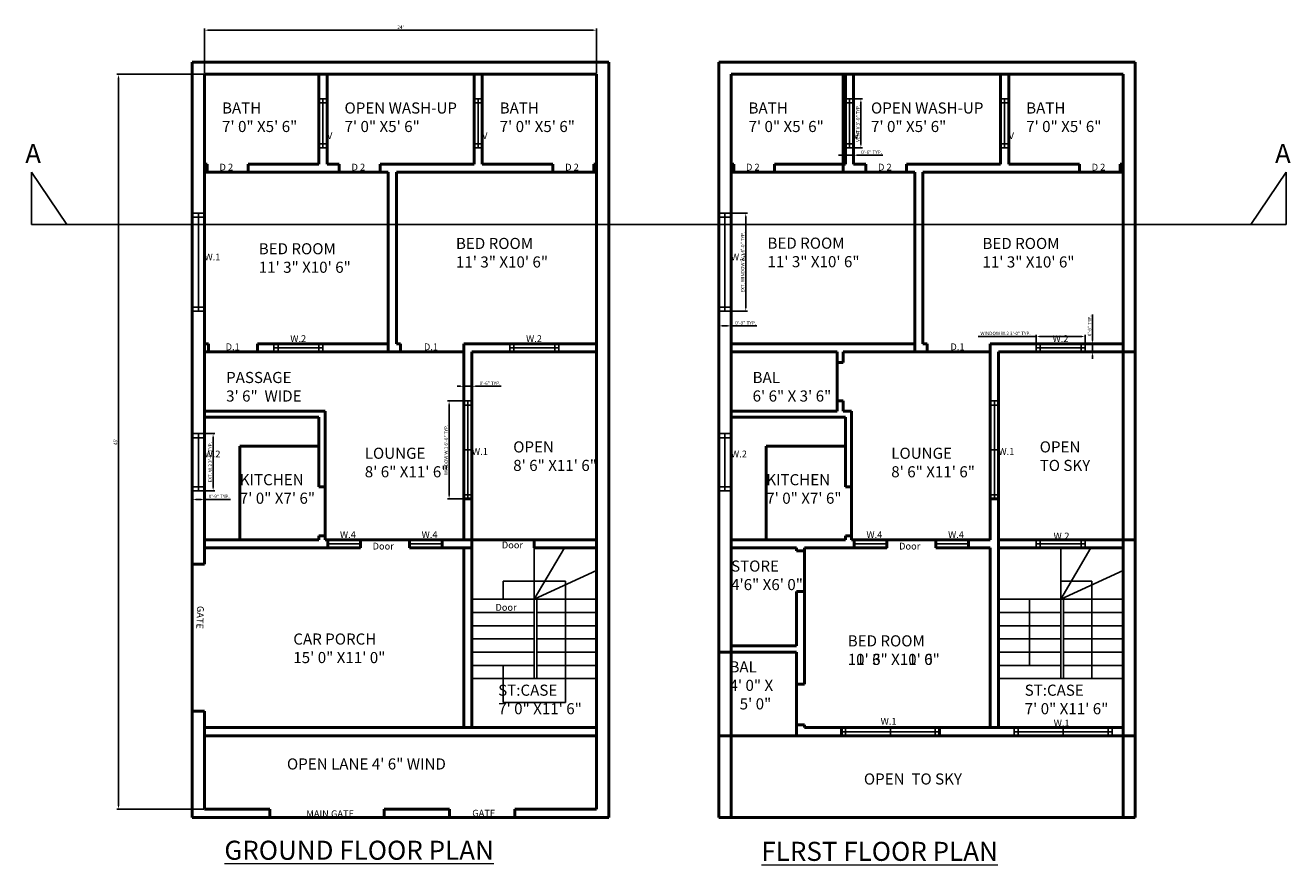
# Model space of a CAD drawing. Units: inches. Extents: x 2117 to 3047, y 1240 to 2266.
# Tile 1 of 4: x 2117 to 3047, y 1240 to 1856. Entities that reach past the tile are written whole.
import ezdxf

# ---------------------------------------------------------------- set-up
doc = ezdxf.new("R2010")
doc.units = ezdxf.units.IN
for name, color, linetype, lineweight in [('A-ANNO-DIMS', 2, 'Continuous', 18), ('A-ANNO-SYMB', 1, 'Continuous', 25), ('A-ANNO-TEXT', 7, 'Continuous', 18), ('A-AREA-IDEN', 3, 'Continuous', 18), ('A-FLOR-STRS', 51, 'Continuous', 25), ('A-GLAZ', 4, 'Continuous', 25), ('A-WALL', 7, 'Continuous', 50)]:
    doc.layers.add(name, color=color, linetype=linetype, lineweight=lineweight)
doc.styles.get("Standard").update_dxf_attribs({"font": 'arial.ttf'})
doc.dimstyles.new('ISO-25', dxfattribs={"dimtxt": 2.5, "dimasz": 2.5, "dimexe": 1.25, "dimexo": 0.625, "dimtad": 1, "dimdec": 1, "dimlunit": 3, "dimtxsty": 'Standard', "dimcen": 2.5, "dimadec": 0, "dimazin": 0, "dimtfac": 1, "dimtdec": 1, "dimtmove": 0, "dimatfit": 3, "dimfxl": 1, "dimarcsym": 0})

# ---------------------------------------------------------------- blocks, each defined once
blk = doc.blocks.new('*D1')
at = {"layer": 'A-ANNO-DIMS', "color": 0, "lineweight": -2, "transparency": 16777216}
for p, q in [((2249.01, 1820.83), (2249.01, 1853.88)), ((2534.51, 1852.63), (2251.51, 1852.63)), ((2537.01, 1820.83), (2537.01, 1853.88))]:
    blk.add_line(p, q, dxfattribs=at)
at = {"layer": 'A-ANNO-DIMS', "color": 0, "transparency": 16777216}
for points in [[(2251.51, 1853.05), (2251.51, 1852.21), (2249.01, 1852.63)], [(2534.51, 1853.05), (2534.51, 1852.21), (2537.01, 1852.63)]]:
    blk.add_solid(points, dxfattribs=at)
at = {"layer": 'Defpoints', "color": 0, "transparency": 16777216}
for p in [(2249.01, 1852.63), (2249.01, 1820.2), (2537.01, 1820.2)]:
    blk.add_point(p, dxfattribs=at)
at = {"layer": 'A-ANNO-DIMS', "color": 0, "transparency": 16777216, "insert": (2393.01, 1854.51), "char_height": 2.5, "attachment_point": 5}
blk.add_mtext("24'", dxfattribs=at)
blk = doc.blocks.new('*D2')
at = {"layer": 'A-ANNO-DIMS', "color": 0, "lineweight": -2, "transparency": 16777216}
for p, q in [((2248.39, 1820.2), (2184.53, 1820.2)), ((2185.78, 1817.7), (2185.78, 1282.7)), ((2248.39, 1280.2), (2184.53, 1280.2))]:
    blk.add_line(p, q, dxfattribs=at)
at = {"layer": 'A-ANNO-DIMS', "color": 0, "transparency": 16777216}
for points in [[(2185.36, 1817.7), (2186.19, 1817.7), (2185.78, 1820.2)], [(2185.36, 1282.7), (2186.19, 1282.7), (2185.78, 1280.2)]]:
    blk.add_solid(points, dxfattribs=at)
at = {"layer": 'Defpoints', "color": 0, "transparency": 16777216}
for p in [(2249.01, 1820.2), (2185.78, 1280.2), (2249.01, 1280.2)]:
    blk.add_point(p, dxfattribs=at)
at = {"layer": 'A-ANNO-DIMS', "color": 0, "transparency": 16777216, "insert": (2183.88, 1550.2), "char_height": 2.5, "attachment_point": 5, "rotation": 90}
blk.add_mtext("45'", dxfattribs=at)
blk = doc.blocks.new('WIN-36')
for p, q in [((0, 36), (6, 36)), ((6, 36), (0, 36)), ((0, 36), (0, 36)), ((0, 36), (6, 36)), ((6, 33), (0, 33)), ((6, 36), (6, 33)), ((0, 0), (0, 3)), ((0, 3), (6, 3)), ((6, 3), (6, 0)), ((0, 0), (6, 0)), ((6, 0), (0, 0))]:
    blk.add_line(p, q)
blk.add_lwpolyline([(6, 36), (0, 36), (0, 0), (6, 0)], close=True)
blk = doc.blocks.new('WIN-36-B')
for p, q in [((6, 36), (0, 36)), ((0, 36), (0, 36)), ((0, 36), (6, 36)), ((6, 33), (0, 33)), ((6, 36), (6, 33)), ((0, 0), (0, 3)), ((0, 3), (6, 3)), ((6, 3), (6, 0)), ((6, 0), (0, 0))]:
    blk.add_line(p, q)
blk.add_lwpolyline([(6, 36), (0, 36), (0, 0), (6, 0)], close=True)
blk = doc.blocks.new('WIN-72')
for p, q in [((0, 72), (6, 72)), ((6, 72), (0, 72)), ((0, 72), (0, 72)), ((0, 72), (6, 72)), ((6, 69), (0, 69)), ((6, 72), (6, 69)), ((0, 36), (0, 39)), ((6, 39), (6, 36)), ((6, 36), (0, 36)), ((6, 36), (0, 36)), ((0, 36), (0, 36)), ((6, 36), (6, 33))]:
    blk.add_line(p, q)
for points in [[(6, 72), (0, 72), (0, 36), (6, 36)], [(6, 36), (0, 36), (0, 0), (6, 0)]]:
    blk.add_lwpolyline(points, close=True)
blk = doc.blocks.new('WIN-72-EXT')
for p, q in [((9, 72), (0, 72)), ((6, 72), (0, 72)), ((0, 72), (0, 72)), ((0, 72), (6, 72)), ((0, 72), (0, 69)), ((0, 69), (9, 69)), ((0, 0), (0, 3)), ((0, 3), (9, 3)), ((9, 0), (0, 0))]:
    blk.add_line(p, q)
blk.add_lwpolyline([(9, 72), (0, 72), (0, 0), (9, 0)], close=True)
blk = doc.blocks.new('WIN-42-EXT')
for p, q in [((0, 42), (9, 42)), ((9, 39), (0, 39)), ((9, 42), (9, 39)), ((9, 3), (0, 3)), ((9, 0), (9, 3)), ((0, 0), (9, 0))]:
    blk.add_line(p, q)
blk.add_lwpolyline([(0, 42), (9, 42), (9, 0), (0, 0)], close=True)
blk = doc.blocks.new('*D20')
at = {"layer": 'A-ANNO-DIMS', "color": 0, "lineweight": -2, "transparency": 16777216}
for p, q in [((2860.11, 1627.6), (2817.55, 1627.6)), ((2860.11, 1622.83), (2860.11, 1628.85)), ((2893.61, 1627.6), (2862.61, 1627.6)), ((2896.11, 1622.83), (2896.11, 1628.85))]:
    blk.add_line(p, q, dxfattribs=at)
at = {"layer": 'A-ANNO-DIMS', "color": 0, "transparency": 16777216}
for points in [[(2862.61, 1628.02), (2862.61, 1627.18), (2860.11, 1627.6)], [(2893.61, 1628.02), (2893.61, 1627.18), (2896.11, 1627.6)]]:
    blk.add_solid(points, dxfattribs=at)
at = {"layer": 'Defpoints', "color": 0, "transparency": 16777216}
for p in [(2860.11, 1627.6), (2860.11, 1622.2), (2896.11, 1622.2)]:
    blk.add_point(p, dxfattribs=at)
at = {"layer": 'A-ANNO-DIMS', "color": 0, "transparency": 16777216, "insert": (2837.58, 1629.52), "char_height": 2.5, "attachment_point": 5}
blk.add_mtext('WINDOW W.2 3\'-0" TYP.', dxfattribs=at)
blk = doc.blocks.new('*D21')
at = {"layer": 'A-ANNO-DIMS', "color": 0, "lineweight": -2, "transparency": 16777216}
for p, q in [((2901.51, 1624.7), (2901.51, 1643.69)), ((2896.74, 1622.2), (2902.76, 1622.2)), ((2901.51, 1616.2), (2901.51, 1622.2)), ((2896.74, 1616.2), (2902.76, 1616.2)), ((2901.51, 1613.7), (2901.51, 1611.2))]:
    blk.add_line(p, q, dxfattribs=at)
at = {"layer": 'A-ANNO-DIMS', "color": 0, "transparency": 16777216}
for points in [[(2901.1, 1624.7), (2901.93, 1624.7), (2901.51, 1622.2)], [(2901.1, 1613.7), (2901.93, 1613.7), (2901.51, 1616.2)]]:
    blk.add_solid(points, dxfattribs=at)
at = {"layer": 'Defpoints', "color": 0, "transparency": 16777216}
for p in [(2896.11, 1622.2), (2901.51, 1622.2), (2896.11, 1616.2)]:
    blk.add_point(p, dxfattribs=at)
at = {"layer": 'A-ANNO-DIMS', "color": 0, "transparency": 16777216, "insert": (2899.61, 1635.45), "char_height": 2.5, "attachment_point": 5, "rotation": 90}
blk.add_mtext('0\'-6" TYP.', dxfattribs=at)
blk = doc.blocks.new('*D22')
at = {"layer": 'A-ANNO-DIMS', "color": 0, "lineweight": -2, "transparency": 16777216}
for p, q in [((2726.49, 1802.2), (2732.51, 1802.2)), ((2731.26, 1768.7), (2731.26, 1799.7)), ((2726.49, 1766.2), (2732.51, 1766.2))]:
    blk.add_line(p, q, dxfattribs=at)
at = {"layer": 'A-ANNO-DIMS', "color": 0, "transparency": 16777216}
for points in [[(2730.85, 1799.7), (2731.68, 1799.7), (2731.26, 1802.2)], [(2730.85, 1768.7), (2731.68, 1768.7), (2731.26, 1766.2)]]:
    blk.add_solid(points, dxfattribs=at)
at = {"layer": 'Defpoints', "color": 0, "transparency": 16777216}
for p in [(2725.86, 1802.2), (2731.26, 1802.2), (2725.86, 1766.2)]:
    blk.add_point(p, dxfattribs=at)
at = {"layer": 'A-ANNO-DIMS', "color": 0, "transparency": 16777216, "insert": (2729.36, 1784.2), "char_height": 2.5, "attachment_point": 5, "rotation": 90}
blk.add_mtext('VENT V 3\'-0" TYP.', dxfattribs=at)
blk = doc.blocks.new('*D23')
at = {"layer": 'A-ANNO-DIMS', "color": 0, "lineweight": -2, "transparency": 16777216}
for p, q in [((2717.36, 1760.8), (2714.86, 1760.8)), ((2719.86, 1765.58), (2719.86, 1759.55)), ((2719.86, 1760.8), (2725.86, 1760.8)), ((2725.86, 1765.58), (2725.86, 1759.55)), ((2728.36, 1760.8), (2747.35, 1760.8))]:
    blk.add_line(p, q, dxfattribs=at)
at = {"layer": 'A-ANNO-DIMS', "color": 0, "transparency": 16777216}
for points in [[(2717.36, 1761.22), (2717.36, 1760.38), (2719.86, 1760.8)], [(2728.36, 1761.22), (2728.36, 1760.38), (2725.86, 1760.8)]]:
    blk.add_solid(points, dxfattribs=at)
at = {"layer": 'Defpoints', "color": 0, "transparency": 16777216}
for p in [(2719.86, 1766.2), (2725.86, 1766.2), (2725.86, 1760.8)]:
    blk.add_point(p, dxfattribs=at)
at = {"layer": 'A-ANNO-DIMS', "color": 0, "transparency": 16777216, "insert": (2739.11, 1762.7), "char_height": 2.5, "attachment_point": 5}
blk.add_mtext('0\'-6" TYP.', dxfattribs=at)
blk = doc.blocks.new('*D24')
at = {"layer": 'A-ANNO-DIMS', "color": 0, "lineweight": -2, "transparency": 16777216}
for p, q in [((2438.89, 1580.2), (2427.46, 1580.2)), ((2428.71, 1510.7), (2428.71, 1577.7)), ((2438.89, 1508.2), (2427.46, 1508.2))]:
    blk.add_line(p, q, dxfattribs=at)
at = {"layer": 'A-ANNO-DIMS', "color": 0, "transparency": 16777216}
for points in [[(2428.3, 1577.7), (2429.13, 1577.7), (2428.71, 1580.2)], [(2428.3, 1510.7), (2429.13, 1510.7), (2428.71, 1508.2)]]:
    blk.add_solid(points, dxfattribs=at)
at = {"layer": 'Defpoints', "color": 0, "transparency": 16777216}
for p in [(2428.71, 1580.2), (2439.51, 1580.2), (2439.51, 1508.2)]:
    blk.add_point(p, dxfattribs=at)
at = {"layer": 'A-ANNO-DIMS', "color": 0, "transparency": 16777216, "insert": (2426.8, 1544.2), "char_height": 2.5, "attachment_point": 5, "rotation": 90}
blk.add_mtext('WINDOW W.1 6\'-0" TYP.', dxfattribs=at)
blk = doc.blocks.new('*D25')
at = {"layer": 'A-ANNO-DIMS', "color": 0, "lineweight": -2, "transparency": 16777216}
for p, q in [((2437.01, 1591), (2434.51, 1591)), ((2439.51, 1580.83), (2439.51, 1592.25)), ((2439.51, 1591), (2445.51, 1591)), ((2445.51, 1580.83), (2445.51, 1592.25)), ((2448.01, 1591), (2467, 1591))]:
    blk.add_line(p, q, dxfattribs=at)
at = {"layer": 'A-ANNO-DIMS', "color": 0, "transparency": 16777216}
for points in [[(2437.01, 1591.42), (2437.01, 1590.58), (2439.51, 1591)], [(2448.01, 1591.42), (2448.01, 1590.58), (2445.51, 1591)]]:
    blk.add_solid(points, dxfattribs=at)
at = {"layer": 'Defpoints', "color": 0, "transparency": 16777216}
for p in [(2445.51, 1591), (2439.51, 1580.2), (2445.51, 1580.2)]:
    blk.add_point(p, dxfattribs=at)
at = {"layer": 'A-ANNO-DIMS', "color": 0, "transparency": 16777216, "insert": (2458.76, 1592.9), "char_height": 2.5, "attachment_point": 5}
blk.add_mtext('0\'-6" TYP.', dxfattribs=at)
blk = doc.blocks.new('*D26')
at = {"layer": 'A-ANNO-DIMS', "color": 0, "lineweight": -2, "transparency": 16777216}
for p, q in [((2636.49, 1718.2), (2647.91, 1718.2)), ((2646.66, 1648.7), (2646.66, 1715.7)), ((2636.49, 1646.2), (2647.91, 1646.2))]:
    blk.add_line(p, q, dxfattribs=at)
at = {"layer": 'A-ANNO-DIMS', "color": 0, "transparency": 16777216}
for points in [[(2646.25, 1715.7), (2647.08, 1715.7), (2646.66, 1718.2)], [(2646.25, 1648.7), (2647.08, 1648.7), (2646.66, 1646.2)]]:
    blk.add_solid(points, dxfattribs=at)
at = {"layer": 'Defpoints', "color": 0, "transparency": 16777216}
for p in [(2635.86, 1718.2), (2646.66, 1718.2), (2635.86, 1646.2)]:
    blk.add_point(p, dxfattribs=at)
at = {"layer": 'A-ANNO-DIMS', "color": 0, "transparency": 16777216, "insert": (2644.74, 1682.2), "char_height": 2.5, "attachment_point": 5, "rotation": 90}
blk.add_mtext('EXT. WINDOW W.1 6\'-0" TYP.', dxfattribs=at)
blk = doc.blocks.new('*D27')
at = {"layer": 'A-ANNO-DIMS', "color": 0, "lineweight": -2, "transparency": 16777216}
for p, q in [((2626.86, 1645.58), (2626.86, 1634.15)), ((2635.86, 1645.58), (2635.86, 1634.15)), ((2629.36, 1635.4), (2633.36, 1635.4)), ((2635.86, 1635.4), (2654.85, 1635.4))]:
    blk.add_line(p, q, dxfattribs=at)
at = {"layer": 'A-ANNO-DIMS', "color": 0, "transparency": 16777216}
for points in [[(2629.36, 1635.82), (2629.36, 1634.98), (2626.86, 1635.4)], [(2633.36, 1635.82), (2633.36, 1634.98), (2635.86, 1635.4)]]:
    blk.add_solid(points, dxfattribs=at)
at = {"layer": 'Defpoints', "color": 0, "transparency": 16777216}
for p in [(2626.86, 1646.2), (2635.86, 1646.2), (2635.86, 1635.4)]:
    blk.add_point(p, dxfattribs=at)
at = {"layer": 'A-ANNO-DIMS', "color": 0, "transparency": 16777216, "insert": (2646.61, 1637.3), "char_height": 2.5, "attachment_point": 5}
blk.add_mtext('0\'-9" TYP.', dxfattribs=at)
blk = doc.blocks.new('*D28')
at = {"layer": 'A-ANNO-DIMS', "color": 0, "lineweight": -2, "transparency": 16777216}
for p, q in [((2249.64, 1556.2), (2256.56, 1556.2)), ((2255.31, 1516.7), (2255.31, 1553.7)), ((2249.64, 1514.2), (2256.56, 1514.2))]:
    blk.add_line(p, q, dxfattribs=at)
at = {"layer": 'A-ANNO-DIMS', "color": 0, "transparency": 16777216}
for points in [[(2254.9, 1553.7), (2255.73, 1553.7), (2255.31, 1556.2)], [(2254.9, 1516.7), (2255.73, 1516.7), (2255.31, 1514.2)]]:
    blk.add_solid(points, dxfattribs=at)
at = {"layer": 'Defpoints', "color": 0, "transparency": 16777216}
for p in [(2249.01, 1556.2), (2255.31, 1556.2), (2249.01, 1514.2)]:
    blk.add_point(p, dxfattribs=at)
at = {"layer": 'A-ANNO-DIMS', "color": 0, "transparency": 16777216, "insert": (2253.41, 1535.2), "char_height": 2.5, "attachment_point": 5, "rotation": 90}
blk.add_mtext('EXT. W.2 3\'-6" TYP.', dxfattribs=at)
blk = doc.blocks.new('*D29')
at = {"layer": 'A-ANNO-DIMS', "color": 0, "lineweight": -2, "transparency": 16777216}
for p, q in [((2240.01, 1513.58), (2240.01, 1506.65)), ((2242.51, 1507.9), (2246.51, 1507.9)), ((2249.01, 1513.58), (2249.01, 1506.65)), ((2249.01, 1507.9), (2268, 1507.9))]:
    blk.add_line(p, q, dxfattribs=at)
at = {"layer": 'A-ANNO-DIMS', "color": 0, "transparency": 16777216}
for points in [[(2242.51, 1508.32), (2242.51, 1507.48), (2240.01, 1507.9)], [(2246.51, 1508.32), (2246.51, 1507.48), (2249.01, 1507.9)]]:
    blk.add_solid(points, dxfattribs=at)
at = {"layer": 'Defpoints', "color": 0, "transparency": 16777216}
for p in [(2240.01, 1514.2), (2249.01, 1514.2), (2249.01, 1507.9)]:
    blk.add_point(p, dxfattribs=at)
at = {"layer": 'A-ANNO-DIMS', "color": 0, "transparency": 16777216, "insert": (2259.76, 1509.8), "char_height": 2.5, "attachment_point": 5}
blk.add_mtext('0\'-9" TYP.', dxfattribs=at)

msp = doc.modelspace()

# ---------------------------------------------------------------- linework, layer by layer
at = {"layer": 'A-ANNO-SYMB'}
for p, q in [((2121.91, 1709.98), (2121.91, 1748.42)), ((2121.91, 1748.42), (2147.8, 1709.98)), ((3043.73, 1748.42), (3017.83, 1709.98)), ((3043.73, 1709.98), (3043.73, 1748.42)), ((2121.91, 1709.98), (3043.73, 1709.98))]:
    msp.add_line(p, q, dxfattribs=at)
at = {"layer": 'A-FLOR-STRS'}
for p, q in [((2491.26, 1472.2), (2491.26, 1376.2)), ((2491.26, 1434.53), (2513.47, 1472.2)), ((2878.11, 1472.2), (2878.11, 1376.2)), ((2878.11, 1434.53), (2900.32, 1472.2)), ((2491.26, 1434.53), (2537.01, 1455.77)), ((2878.11, 1434.53), (2923.86, 1455.77)), ((2468.39, 1434.53), (2468.39, 1447.73)), ((2468.39, 1447.73), (2514.12, 1447.73)), ((2514.12, 1447.73), (2514.12, 1358.7)), ((2878.11, 1447.73), (2900.96, 1447.73)), ((2900.96, 1447.73), (2900.96, 1376.2)), ((2445.51, 1434.53), (2537.01, 1434.53)), ((2493.26, 1434.53), (2493.26, 1376.2)), ((2832.36, 1434.53), (2923.86, 1434.53)), ((2855.24, 1385.92), (2855.24, 1434.53)), ((2880.11, 1434.53), (2880.11, 1376.2)), ((2445.51, 1424.81), (2491.26, 1424.81)), ((2493.26, 1424.81), (2537.01, 1424.81)), ((2832.36, 1424.81), (2878.11, 1424.81)), ((2880.11, 1424.81), (2923.86, 1424.81)), ((2445.51, 1415.09), (2491.26, 1415.09)), ((2493.26, 1415.09), (2537.01, 1415.09)), ((2832.36, 1415.09), (2878.11, 1415.09)), ((2880.11, 1415.09), (2923.86, 1415.09)), ((2445.51, 1405.37), (2491.26, 1405.37)), ((2493.26, 1405.37), (2537.01, 1405.37)), ((2832.36, 1405.37), (2878.11, 1405.37)), ((2880.11, 1405.37), (2923.86, 1405.37)), ((2445.51, 1395.64), (2491.26, 1395.64)), ((2493.26, 1395.64), (2537.01, 1395.64)), ((2832.36, 1395.64), (2878.11, 1395.64)), ((2880.11, 1395.64), (2923.86, 1395.64)), ((2445.51, 1385.92), (2491.26, 1385.92)), ((2468.39, 1358.7), (2468.39, 1385.92)), ((2493.26, 1385.92), (2537.01, 1385.92)), ((2832.36, 1385.92), (2878.11, 1385.92)), ((2880.11, 1385.92), (2923.86, 1385.92)), ((2445.51, 1376.2), (2537.01, 1376.2)), ((2832.36, 1376.2), (2923.86, 1376.2)), ((2514.12, 1358.7), (2468.39, 1358.7))]:
    msp.add_line(p, q, dxfattribs=at)
at = {"layer": 'A-GLAZ'}
for p, q in [((2336.01, 1802.2), (2336.01, 1766.2)), ((2450.01, 1802.2), (2450.01, 1766.2)), ((2722.86, 1802.2), (2722.86, 1766.2)), ((2836.86, 1802.2), (2836.86, 1766.2)), ((2244.51, 1718.2), (2244.51, 1646.2)), ((2631.36, 1718.2), (2631.36, 1646.2)), ((2240.01, 1682.2), (2240.01, 1685.2)), ((2626.86, 1682.2), (2626.86, 1685.2)), ((2300.01, 1619.2), (2336.01, 1619.2)), ((2473.26, 1619.2), (2509.26, 1619.2)), ((2860.11, 1619.2), (2896.11, 1619.2)), ((2442.51, 1580.2), (2442.51, 1544.2)), ((2829.36, 1580.2), (2829.36, 1541.15)), ((2244.51, 1556.2), (2244.51, 1514.2)), ((2631.36, 1556.2), (2631.36, 1514.2)), ((2442.51, 1544.2), (2442.51, 1508.2)), ((2829.36, 1544.2), (2829.36, 1508.2)), ((2439.51, 1508.2), (2439.51, 1511.2)), ((2439.51, 1511.2), (2445.51, 1511.2)), ((2445.51, 1511.2), (2445.51, 1508.2)), ((2826.36, 1508.2), (2826.36, 1511.2)), ((2826.36, 1511.2), (2832.36, 1511.2)), ((2832.36, 1511.2), (2832.36, 1508.2)), ((2339.51, 1475.2), (2363.51, 1475.2)), ((2399.51, 1472.2), (2399.51, 1475.2)), ((2399.51, 1475.2), (2423.51, 1475.2)), ((2726.36, 1475.2), (2750.36, 1475.2)), ((2786.36, 1472.2), (2786.36, 1475.2)), ((2786.36, 1475.2), (2810.36, 1475.2)), ((2860.11, 1475.2), (2896.11, 1475.2)), ((2719.94, 1340.2), (2719.94, 1334.2)), ((2752.94, 1340.2), (2755.94, 1340.2)), ((2785.94, 1334.2), (2785.94, 1340.2)), ((2846.92, 1340.2), (2846.92, 1334.2)), ((2879.92, 1340.2), (2882.92, 1340.2)), ((2912.92, 1334.2), (2912.92, 1340.2)), ((2752.94, 1337.2), (2716.94, 1337.2)), ((2788.94, 1337.2), (2749.89, 1337.2)), ((2879.92, 1337.2), (2843.92, 1337.2)), ((2915.92, 1337.2), (2876.86, 1337.2))]:
    msp.add_line(p, q, dxfattribs=at)
for points in [[(2339.51, 1472.2), (2363.51, 1472.2), (2363.51, 1478.2), (2339.51, 1478.2)], [(2399.51, 1472.2), (2423.51, 1472.2), (2423.51, 1478.2), (2399.51, 1478.2)], [(2726.36, 1472.2), (2750.36, 1472.2), (2750.36, 1478.2), (2726.36, 1478.2)], [(2786.36, 1472.2), (2810.36, 1472.2), (2810.36, 1478.2), (2786.36, 1478.2)], [(2752.94, 1334.2), (2752.94, 1340.2), (2716.94, 1340.2), (2716.94, 1334.2)], [(2788.94, 1334.2), (2788.94, 1340.2), (2752.94, 1340.2), (2752.94, 1334.2)], [(2879.92, 1334.2), (2879.92, 1340.2), (2843.92, 1340.2), (2843.92, 1334.2)], [(2915.92, 1334.2), (2915.92, 1340.2), (2879.92, 1340.2), (2879.92, 1334.2)]]:
    msp.add_lwpolyline(points, close=True, dxfattribs=at)
at = {"layer": 'A-WALL'}
for p, q in [((2240.01, 1829.2), (2240.01, 1274.2)), ((2240.01, 1829.2), (2546.01, 1829.2)), ((2546.01, 1829.2), (2546.01, 1274.2)), ((2626.86, 1829.2), (2626.86, 1274.2)), ((2626.86, 1829.2), (2932.86, 1829.2)), ((2626.86, 1829.2), (2626.86, 1274.2)), ((2932.86, 1829.2), (2932.86, 1274.2)), ((2932.86, 1829.2), (2932.86, 1274.2)), ((2249.01, 1820.2), (2537.01, 1820.2)), ((2249.01, 1820.2), (2249.01, 1460.2)), ((2333.01, 1820.2), (2333.01, 1754.2)), ((2339.01, 1820.2), (2339.01, 1754.2)), ((2447.01, 1820.2), (2447.01, 1754.2)), ((2453.01, 1820.2), (2453.01, 1754.2)), ((2537.01, 1820.2), (2537.01, 1280.2)), ((2635.86, 1820.2), (2635.86, 1395.7)), ((2635.86, 1820.2), (2923.86, 1820.2)), ((2635.86, 1820.2), (2635.86, 1274.2)), ((2718.36, 1820.2), (2718.36, 1748.2)), ((2719.86, 1820.2), (2719.86, 1754.2)), ((2725.86, 1820.2), (2725.86, 1754.2)), ((2833.86, 1820.2), (2833.86, 1754.2)), ((2839.86, 1820.2), (2839.86, 1754.2)), ((2923.86, 1754.2), (2923.86, 1820.2)), ((2923.86, 1820.2), (2923.86, 1274.2)), ((2249.01, 1754.2), (2251.01, 1754.2)), ((2249.01, 1748.2), (2251.01, 1748.2)), ((2251.01, 1754.2), (2251.01, 1748.2)), ((2251.01, 1748.2), (2378.01, 1748.2)), ((2281.01, 1754.2), (2281.01, 1748.2)), ((2281.01, 1754.2), (2333.01, 1754.2)), ((2339.01, 1754.2), (2348.01, 1754.2)), ((2348.01, 1754.2), (2348.01, 1748.2)), ((2378.01, 1754.2), (2378.01, 1748.2)), ((2378.01, 1754.2), (2447.01, 1754.2)), ((2378.01, 1748.2), (2384.01, 1748.2)), ((2384.01, 1748.2), (2384.01, 1616.2)), ((2390.01, 1748.2), (2390.01, 1622.2)), ((2390.01, 1748.2), (2535.01, 1748.2)), ((2453.01, 1754.2), (2505.01, 1754.2)), ((2505.01, 1754.2), (2505.01, 1748.2)), ((2535.01, 1754.2), (2535.01, 1748.2)), ((2535.01, 1754.2), (2537.01, 1754.2)), ((2535.01, 1748.2), (2537.01, 1748.2)), ((2635.86, 1754.2), (2637.86, 1754.2)), ((2635.86, 1748.2), (2637.86, 1748.2)), ((2637.86, 1754.2), (2637.86, 1748.2)), ((2637.86, 1748.2), (2764.86, 1748.2)), ((2667.86, 1754.2), (2667.86, 1748.2)), ((2667.86, 1754.2), (2719.86, 1754.2)), ((2725.86, 1754.2), (2734.86, 1754.2)), ((2734.86, 1754.2), (2734.86, 1748.2)), ((2764.86, 1754.2), (2764.86, 1748.2)), ((2764.86, 1754.2), (2833.86, 1754.2)), ((2764.86, 1748.2), (2770.86, 1748.2)), ((2770.86, 1748.2), (2770.86, 1616.2)), ((2776.86, 1748.2), (2776.86, 1622.2)), ((2776.86, 1748.2), (2921.86, 1748.2)), ((2839.86, 1754.2), (2891.86, 1754.2)), ((2891.86, 1754.2), (2891.86, 1748.2)), ((2921.86, 1754.2), (2921.86, 1748.2)), ((2921.86, 1754.2), (2923.86, 1754.2)), ((2921.86, 1748.2), (2923.86, 1748.2)), ((2923.86, 1622.2), (2923.86, 1748.2)), ((2249.01, 1622.2), (2252.01, 1622.2)), ((2252.01, 1622.2), (2252.01, 1616.2)), ((2288.01, 1622.2), (2384.01, 1622.2)), ((2288.01, 1622.2), (2288.01, 1616.2)), ((2390.01, 1622.2), (2393.01, 1622.2)), ((2393.01, 1622.2), (2393.01, 1616.2)), ((2439.51, 1622.2), (2439.51, 1478.2)), ((2439.51, 1622.2), (2537.01, 1622.2)), ((2635.86, 1622.2), (2638.86, 1622.2)), ((2638.86, 1622.2), (2770.86, 1622.2)), ((2776.86, 1622.2), (2779.86, 1622.2)), ((2779.86, 1622.2), (2779.86, 1616.2)), ((2826.36, 1622.2), (2826.36, 1478.2)), ((2826.36, 1622.2), (2923.86, 1622.2)), ((2249.01, 1616.2), (2439.51, 1616.2)), ((2445.51, 1616.2), (2445.51, 1340.2)), ((2445.51, 1616.2), (2537.01, 1616.2)), ((2635.86, 1616.2), (2713.86, 1616.2)), ((2713.86, 1616.2), (2713.86, 1572.7)), ((2713.86, 1608.57), (2718.36, 1608.57)), ((2718.36, 1616.2), (2718.36, 1608.57)), ((2718.36, 1616.2), (2826.36, 1616.2)), ((2832.36, 1616.2), (2832.36, 1340.2)), ((2832.36, 1616.2), (2932.86, 1616.2)), ((2249.01, 1572.7), (2337.51, 1572.7)), ((2337.51, 1572.7), (2337.51, 1478.2)), ((2635.86, 1572.7), (2713.86, 1572.7)), ((2713.86, 1580.33), (2718.36, 1580.33)), ((2718.36, 1580.33), (2718.36, 1572.7)), ((2718.36, 1572.7), (2724.36, 1572.7)), ((2724.36, 1572.7), (2724.36, 1478.2)), ((2249.01, 1568.2), (2333.01, 1568.2)), ((2333.01, 1568.2), (2333.01, 1517.2)), ((2635.86, 1568.2), (2719.86, 1568.2)), ((2719.86, 1568.2), (2719.86, 1517.2)), ((2333.01, 1547.12), (2274.89, 1547.12)), ((2274.89, 1547.12), (2274.89, 1478.2)), ((2719.86, 1547.12), (2661.74, 1547.12)), ((2661.74, 1547.12), (2661.74, 1478.2)), ((2333.01, 1517.2), (2337.51, 1517.2)), ((2719.86, 1517.2), (2724.36, 1517.2)), ((2439.51, 1508.2), (2445.51, 1508.2)), ((2445.51, 1508.2), (2439.51, 1508.2)), ((2826.36, 1508.2), (2832.36, 1508.2)), ((2832.36, 1508.2), (2826.36, 1508.2)), ((2333.01, 1481.2), (2337.51, 1481.2)), ((2333.01, 1481.2), (2333.01, 1478.2)), ((2719.86, 1481.2), (2719.86, 1478.2)), ((2719.86, 1481.2), (2724.36, 1481.2)), ((2249.01, 1478.2), (2333.01, 1478.2)), ((2249.01, 1472.2), (2363.51, 1472.2)), ((2337.51, 1478.2), (2363.51, 1478.2)), ((2339.51, 1478.2), (2339.51, 1472.2)), ((2363.51, 1478.2), (2363.51, 1472.2)), ((2363.51, 1478.2), (2399.51, 1478.2)), ((2399.51, 1478.2), (2399.51, 1472.2)), ((2399.51, 1478.2), (2439.51, 1478.2)), ((2399.51, 1478.2), (2537.01, 1478.2)), ((2399.51, 1472.2), (2445.51, 1472.2)), ((2423.51, 1478.2), (2423.51, 1472.2)), ((2439.51, 1472.2), (2439.51, 1340.2)), ((2481.51, 1478.2), (2537.01, 1478.2)), ((2491.26, 1472.2), (2491.26, 1478.2)), ((2491.26, 1472.2), (2537.01, 1472.2)), ((2537.01, 1472.2), (2537.01, 1280.2)), ((2537.01, 1280.2), (2537.01, 1472.2)), ((2537.01, 1472.2), (2537.01, 1472.2)), ((2537.01, 1472.2), (2537.01, 1472.2)), ((2537.01, 1472.2), (2537.01, 1472.2)), ((2537.01, 1472.2), (2537.01, 1472.2)), ((2635.86, 1478.2), (2719.86, 1478.2)), ((2635.86, 1472.2), (2683.86, 1472.2)), ((2683.86, 1472.2), (2683.86, 1470.2)), ((2683.86, 1470.2), (2689.86, 1470.2)), ((2689.86, 1472.2), (2750.36, 1472.2)), ((2689.86, 1472.2), (2689.86, 1372.2)), ((2724.36, 1478.2), (2750.36, 1478.2)), ((2726.36, 1478.2), (2726.36, 1472.2)), ((2750.36, 1478.2), (2750.36, 1472.2)), ((2750.36, 1478.2), (2786.36, 1478.2)), ((2786.36, 1478.2), (2786.36, 1472.2)), ((2786.36, 1478.2), (2826.36, 1478.2)), ((2786.36, 1478.2), (2826.36, 1478.2)), ((2786.36, 1472.2), (2826.36, 1472.2)), ((2810.36, 1478.2), (2810.36, 1472.2)), ((2826.36, 1472.2), (2826.36, 1340.2)), ((2832.36, 1478.2), (2932.86, 1478.2)), ((2878.11, 1472.2), (2832.36, 1472.2)), ((2868.36, 1478.2), (2923.86, 1478.2)), ((2878.11, 1472.2), (2923.86, 1472.2)), ((2923.86, 1472.2), (2923.86, 1340.2)), ((2923.86, 1472.2), (2923.86, 1340.2)), ((2923.86, 1472.2), (2923.86, 1472.2)), ((2923.86, 1472.2), (2923.86, 1472.2)), ((2923.86, 1472.2), (2923.86, 1472.2)), ((2923.86, 1472.2), (2923.86, 1472.2)), ((2240.01, 1460.2), (2249.01, 1460.2)), ((2683.86, 1440.2), (2689.86, 1440.2)), ((2683.86, 1440.2), (2683.86, 1400.2)), ((2626.86, 1395.7), (2683.86, 1395.7)), ((2635.86, 1400.2), (2683.86, 1400.2)), ((2683.86, 1395.7), (2683.86, 1342.2)), ((2689.86, 1395.7), (2689.86, 1372.2)), ((2683.86, 1372.2), (2689.86, 1372.2)), ((2240.01, 1352.2), (2249.01, 1352.2)), ((2249.01, 1352.2), (2249.01, 1280.2)), ((2249.01, 1340.2), (2537.01, 1340.2)), ((2683.86, 1342.2), (2689.86, 1342.2)), ((2683.86, 1342.2), (2683.86, 1340.2)), ((2683.86, 1340.2), (2683.86, 1334.2)), ((2689.86, 1342.2), (2689.86, 1340.2)), ((2689.86, 1340.2), (2923.86, 1340.2)), ((2716.94, 1340.2), (2716.94, 1334.2)), ((2788.94, 1340.2), (2788.94, 1334.2)), ((2249.01, 1334.2), (2537.01, 1334.2)), ((2626.86, 1334.2), (2932.86, 1334.2)), ((2240.01, 1274.2), (2546.01, 1274.2)), ((2249.01, 1280.2), (2297.01, 1280.2)), ((2297.01, 1280.2), (2297.01, 1274.2)), ((2381.01, 1280.2), (2381.01, 1274.2)), ((2381.01, 1280.2), (2429.01, 1280.2)), ((2429.01, 1280.2), (2429.01, 1274.2)), ((2477.01, 1280.2), (2477.01, 1274.2)), ((2477.01, 1280.2), (2537.01, 1280.2)), ((2626.86, 1274.2), (2932.86, 1274.2))]:
    msp.add_line(p, q, dxfattribs=at)

# ---------------------------------------------------------------- block references
at = {"layer": 'A-GLAZ'}
for name, p in [('WIN-36-B', (2333.01, 1766.2)), ('WIN-36', (2447.01, 1766.2)), ('WIN-36-B', (2719.86, 1766.2)), ('WIN-36', (2833.86, 1766.2)), ('WIN-72-EXT', (2240.01, 1646.2)), ('WIN-72-EXT', (2626.86, 1646.2)), ('WIN-72', (2439.51, 1508.2)), ('WIN-72', (2826.36, 1508.2)), ('WIN-42-EXT', (2240.01, 1514.2)), ('WIN-42-EXT', (2626.86, 1514.2))]:
    msp.add_blockref(name, p, dxfattribs=at)
for name, p, rotation in [('WIN-36', (2336.01, 1616.2), 90.00000000000384), ('WIN-36', (2509.26, 1616.2), 89.9999999999994), ('WIN-36', (2896.11, 1616.2), 89.99999999999844), ('WIN-36-B', (2896.11, 1472.2), 89.99999999999584)]:
    msp.add_blockref(name, p, dxfattribs=dict(at, rotation=rotation))

# ---------------------------------------------------------------- texts
at = {"layer": 'A-ANNO-SYMB', "char_height": 14, "attachment_point": 1}
for insert in [(2117.23, 1768.97), (3035.53, 1768.97)]:
    msp.add_mtext_dynamic_manual_height_columns('A', width=20.0741, gutter_width=70, heights=[0], dxfattribs=dict(at, insert=insert))
at = {"layer": 'A-ANNO-TEXT', "attachment_point": 1}
for s, width, gutter_width, heights, insert, char_height in [('V', 5, 25, [6.31], (2339.01, 1777.66), 5), ('V', 5, 25, [6.31], (2453.01, 1777.66), 5), ('V', 5, 25, [6.31], (2725.86, 1777.66), 5), ('V', 5, 25, [6.31], (2839.86, 1777.66), 5), ('D 2', 16.985, 25, [0], (2260, 1754.51), 5), ('D 2', 16.985, 25, [0], (2357, 1754.51), 5), ('D 2', 16.985, 25, [0], (2514, 1754.51), 5), ('D 2', 16.985, 25, [0], (2646.85, 1754.51), 5), ('D 2', 16.985, 25, [0], (2743.85, 1754.51), 5), ('D 2', 16.985, 25, [0], (2900.85, 1754.51), 5), ('W.1', 16.985, 25, [0], (2249, 1688.51), 5), ('W.3', 16.985, 25, [0], (2635.85, 1688.51), 5), ('W.2', 16.985, 25, [0], (2312, 1628.51), 5), ('W.2', 16.985, 25, [0], (2485.25, 1628.51), 5), ('W.2', 16.985, 25, [0], (2872.1, 1628.51), 5), ('D.1', 16.985, 25, [5.02], (2264.51, 1622.51), 5), ('D.1', 16.985, 25, [0], (2410.2, 1622.51), 5), ('D.1', 16.985, 25, [0], (2797.04, 1622.51), 5), ('W.2', 16.985, 25, [0], (2249, 1543.76), 5), ('W.1', 16.985, 25, [0], (2445.51, 1545.59), 5), ('W.2', 16.985, 25, [0], (2635.85, 1543.76), 5), ('W.1', 16.985, 25, [0], (2832.36, 1545.59), 5), ('W.4', 16.985, 25, [0], (2348.5, 1484.51), 5), ('W.4', 16.985, 25, [0], (2408.5, 1484.51), 5), ('W.4', 16.985, 25, [0], (2735.35, 1484.51), 5), ('W.4', 16.985, 25, [0], (2795.35, 1484.51), 5), ('W.2', 16.985, 25, [0], (2872.83, 1483.51), 5), ('Door', 16.985, 25, [0], (2372.47, 1476.07), 5), ('Door', 16.985, 25, [0], (2467.42, 1476.91), 5), ('Door', 16.985, 25, [0], (2759.32, 1476.07), 5), ('Door', 16.985, 25, [0], (2462.72, 1431.07), 5), ('W.1', 16.985, 25, [0], (2745.78, 1347.34), 5), ('W.1', 16.985, 25, [0], (2872.95, 1346.1), 5), ('MAIN GATE', 38.3527, 25, [0], (2323.77, 1279.42), 5), ('GATE', 16.985, 25, [0], (2445.71, 1279.87), 5), ('{\\LGROUND FLOOR PLAN}', 221.8965, 70, [0], (2263.55, 1257.15), 14), ('{\\LFLRST FLOOR PLAN}', 221.8965, 70, [0], (2658.18, 1256.33), 14)]:
    msp.add_mtext_dynamic_manual_height_columns(s, width=width, gutter_width=gutter_width, heights=heights, dxfattribs=dict(at, insert=insert, char_height=char_height))
at = {"layer": 'A-ANNO-TEXT', "insert": (2248.55, 1429.55), "char_height": 5, "attachment_point": 1, "rotation": 268.12064}
msp.add_mtext_dynamic_manual_height_columns('GATE ', width=16.985, gutter_width=25, heights=[0], dxfattribs=at)
at = {"layer": 'A-AREA-IDEN', "char_height": 8.159, "attachment_point": 1}
for s, width, insert in [('BATH \\P7\' 0" X5\' 6"', 161.1385, (2261.84, 1799.55)), ('OPEN WASH-UP \\P7\' 0" X5\' 6"', 161.1385, (2351.84, 1799.55)), ('BATH \\P7\' 0" X5\' 6"', 161.1385, (2465.84, 1799.55)), ('BATH \\P7\' 0" X5\' 6"', 161.1385, (2648.69, 1799.55)), ('OPEN WASH-UP \\P7\' 0" X5\' 6"', 161.1385, (2738.69, 1799.55)), ('BATH \\P7\' 0" X5\' 6"', 161.1385, (2852.69, 1799.55)), ('BED ROOM \\P11\' 3" X10\' 6"', 161.1385, (2288.81, 1696.13)), ('BED ROOM \\P11\' 3" X10\' 6"', 161.1385, (2433.73, 1700.03)), ('BED ROOM \\P11\' 3" X10\' 6"', 161.1385, (2662.62, 1700.24)), ('BED ROOM \\P11\' 3" X10\' 6"', 161.1385, (2820.57, 1700.03)), ('PASSAGE\\P3\' 6"  WIDE', 161.1385, (2264.84, 1601.55)), ('BAL\\P6\' 6" X 3\' 6"  ', 161.1385, (2651.69, 1601.55)), ('LOUNGE \\P8\' 6" X11\' 6"', 161.1385, (2366.72, 1545.88)), ('OPEN\\P8\' 6" X11\' 6"', 161.1385, (2475.8, 1550.55)), ('LOUNGE \\P8\' 6" X11\' 6"', 161.1385, (2753.57, 1545.88)), ('OPEN \\PTO SKY', 161.1385, (2862.65, 1550.55)), ('KITCHEN\\P7\' 0" X7\' 6"', 161.1385, (2274.89, 1526.46)), ('KITCHEN\\P7\' 0" X7\' 6"', 161.1385, (2661.74, 1526.46)), ('STORE\\P4\'6" X6\' 0"', 161.1385, (2635.86, 1463)), ('CAR PORCH\\P15\' 0" X11\' 0"', 161.1385, (2314.22, 1409.39)), ('BED ROOM \\P11\' 3" X10\' 6"', 161.1385, (2721.59, 1408.05)), ('BED ROOM \\P10\' 6" X11\' 0"', 161.1385, (2721.59, 1408.05)), ('BAL\\P4\' 0" X\\P   5\' 0"', 56.416, (2634.7, 1388.96)), ('ST:CASE\\P7\' 0" X11\' 6"', 161.1385, (2464.75, 1371.81)), ('ST:CASE\\P7\' 0" X11\' 6"', 161.1385, (2851.6, 1371.81)), ('OPEN LANE 4\' 6" WIND', 161.1385, (2309.56, 1317.62)), ('OPEN  TO SKY', 92.3899, (2733.47, 1306.58))]:
    msp.add_mtext_dynamic_manual_height_columns(s, width=width, gutter_width=40.8, heights=[0], dxfattribs=dict(at, insert=insert))

# ---------------------------------------------------------------- dimensions: what is measured, and where the dimension line sits
at = {"layer": 'A-ANNO-DIMS'}
dim = msp.add_linear_dim(base=(2249.01, 1852.63), p1=(2537.01, 1820.2), p2=(2249.01, 1820.2), dimstyle='ISO-25', override={"dimclrd": 0, "dimclre": 0, "dimclrt": 0}, dxfattribs=at)
dim.commit()
dim.dimension.update_dxf_attribs({"geometry": '*D1', "text_midpoint": (2393.01, 1854.51)})
dim = msp.add_linear_dim(base=(2185.78, 1280.2), p1=(2249.01, 1820.2), p2=(2249.01, 1280.2), angle=90, dimstyle='ISO-25', override={"dimclrd": 0, "dimclre": 0, "dimclrt": 0}, dxfattribs=at)
dim.commit()
dim.dimension.update_dxf_attribs({"geometry": '*D2', "text_midpoint": (2183.88, 1550.2)})
for base, p1, p2, angle, text, picture, middle in [((2731.26, 1802.2), (2725.86, 1766.2), (2725.86, 1802.2), 90, 'VENT V <> TYP.', '*D22', (2729.36, 1784.2)), ((2646.66, 1718.2), (2635.86, 1646.2), (2635.86, 1718.2), 90, 'EXT. WINDOW W.1 <> TYP.', '*D26', (2644.74, 1682.2)), ((2860.11, 1627.6), (2896.11, 1622.2), (2860.11, 1622.2), 180, 'WINDOW W.2 <> TYP.', '*D20', (2837.58, 1629.52)), ((2901.51, 1622.2), (2896.11, 1616.2), (2896.11, 1622.2), 90, '<> TYP.', '*D21', (2899.61, 1635.45)), ((2428.71, 1580.2), (2439.51, 1508.2), (2439.51, 1580.2), 90, 'WINDOW W.1 <> TYP.', '*D24', (2426.8, 1544.2)), ((2255.31, 1556.2), (2249.01, 1514.2), (2249.01, 1556.2), 90, 'EXT. W.2 <> TYP.', '*D28', (2253.41, 1535.2))]:
    dim = msp.add_linear_dim(base=base, p1=p1, p2=p2, angle=angle, text=text, dimstyle='ISO-25', override={"dimdec": 1, "dimrnd": 0, "dimzin": 1, "dimlunit": 4, "dimfrac": 2}, dxfattribs=at)
    dim.commit()
    dim.dimension.update_dxf_attribs({"geometry": picture, "text_midpoint": middle})
for base, p1, p2, picture, middle in [((2725.86, 1760.8), (2719.86, 1766.2), (2725.86, 1766.2), '*D23', (2739.11, 1762.7)), ((2635.86, 1635.4), (2626.86, 1646.2), (2635.86, 1646.2), '*D27', (2646.61, 1637.3)), ((2445.51, 1591), (2439.51, 1580.2), (2445.51, 1580.2), '*D25', (2458.76, 1592.9)), ((2249.01, 1507.9), (2240.01, 1514.2), (2249.01, 1514.2), '*D29', (2259.76, 1509.8))]:
    dim = msp.add_linear_dim(base=base, p1=p1, p2=p2, text='<> TYP.', dimstyle='ISO-25', override={"dimdec": 1, "dimrnd": 0, "dimzin": 1, "dimlunit": 4, "dimfrac": 2}, dxfattribs=at)
    dim.commit()
    dim.dimension.update_dxf_attribs({"geometry": picture, "text_midpoint": middle})

doc.saveas('drawing.dxf')
